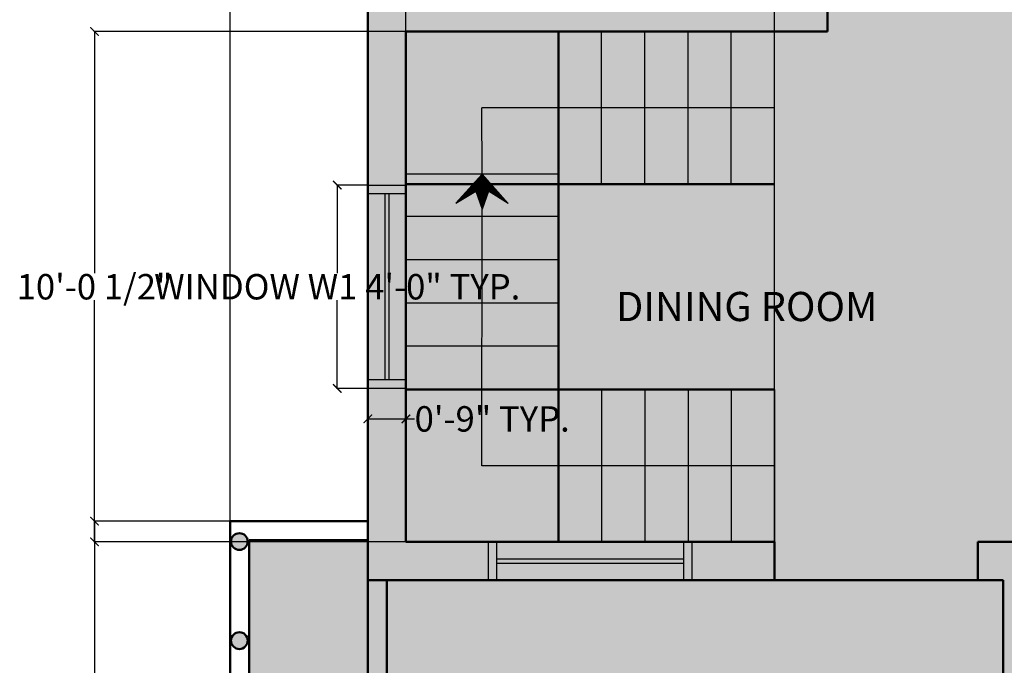
# Model space of a CAD drawing. Units: inches. Extents: x 528 to 2620, y -1066 to 798.
# Tile 22 of 41: x 975 to 1207, y 371 to 524. Entities that reach past the tile are written whole.
import ezdxf

# ---------------------------------------------------------------- set-up
doc = ezdxf.new("R2010")
doc.units = ezdxf.units.IN
doc.header["$MEASUREMENT"] = 0
for name, color, linetype, lineweight in [('A-ANNO-DIMS', 2, 'Continuous', 18), ('A-AREA-IDEN', 7, 'Continuous', 18), ('A-FLOR-STRS', 6, 'Continuous', 25), ('A-GLAZ', 3, 'Continuous', 25), ('A-WALL', 7, 'Continuous', 50), ('A-WALL-PATT', 8, 'Continuous', 13)]:
    doc.layers.add(name, color=color, linetype=linetype, lineweight=lineweight)
doc.styles.get("Standard").update_dxf_attribs({"font": 'arial.ttf'})
doc.dimstyles.get("Standard").update_dxf_attribs({"dimtxt": 6, "dimasz": 2, "dimexe": 0.18, "dimexo": 0.0625, "dimgap": 0.09, "dimtad": 0, "dimtih": 1, "dimtoh": 1, "dimdec": 1, "dimzin": 0, "dimdsep": 46, "dimlunit": 3, "dimtxsty": 'Standard', "dimblk": 'ARCHTICK', "dimcen": 0.09, "dimadec": 0, "dimazin": 0, "dimtfac": 1, "dimtdec": 1, "dimtofl": 0, "dimtmove": 0, "dimatfit": 3, "dimfxl": 1, "dimtolj": 1, "dimtzin": 0, "dimarcsym": 0})

# ---------------------------------------------------------------- blocks, each defined once
blk = doc.blocks.new('WIN-1200')
for p, q in [((677.56, 718.92), (725.56, 718.92)), ((677.56, 709.92), (677.56, 718.92)), ((679.56, 709.92), (679.56, 718.92)), ((723.56, 718.92), (723.56, 709.92)), ((725.56, 718.92), (725.56, 709.92)), ((679.56, 714.92), (723.56, 714.92)), ((679.56, 713.92), (723.56, 713.92)), ((725.56, 709.92), (677.56, 709.92))]:
    blk.add_line(p, q)
blk = doc.blocks.new('_ArchTick')
at = {"color": 0, "linetype": 'ByBlock', "const_width": 0.15}
blk.add_lwpolyline([(-0.5, -0.5), (0.5, 0.5)], dxfattribs=at)
blk = doc.blocks.new('*D50')
at = {"layer": 'A-ANNO-DIMS', "color": 0, "lineweight": -2, "transparency": 16777216}
for p, q in [((1056.93, 484.67), (1049.62, 484.67)), ((1049.8, 484.67), (1049.8, 463.87)), ((1049.8, 436.67), (1049.8, 457.48)), ((1056.93, 436.67), (1049.62, 436.67))]:
    blk.add_line(p, q, dxfattribs=at)
at = {"layer": 'Defpoints', "color": 0, "transparency": 16777216}
for p in [(1057, 484.67), (1049.8, 436.67), (1057, 436.67)]:
    blk.add_point(p, dxfattribs=at)
at = {"layer": 'A-ANNO-DIMS', "color": 0, "lineweight": -2, "transparency": 16777216, "xscale": 2, "yscale": 2, "zscale": 2}
for p, rotation in [((1049.8, 484.67), 90), ((1049.8, 436.67), 270)]:
    blk.add_blockref('_ArchTick', p, dxfattribs=dict(at, rotation=rotation))
at = {"layer": 'A-ANNO-DIMS', "color": 0, "transparency": 16777216, "insert": (1049.8, 460.67), "char_height": 6, "attachment_point": 5}
blk.add_mtext('\\A1;WINDOW W1 4\'-0" TYP.', dxfattribs=at)
blk = doc.blocks.new('*D51')
at = {"layer": 'A-ANNO-DIMS', "color": 0, "lineweight": -2, "transparency": 16777216}
for p, q in [((1057, 436.61), (1057, 429.29)), ((1066, 436.61), (1066, 429.29)), ((1057, 429.47), (1066, 429.47)), ((1066, 429.47), (1068, 429.47))]:
    blk.add_line(p, q, dxfattribs=at)
at = {"layer": 'Defpoints', "color": 0, "transparency": 16777216}
for p in [(1057, 436.67), (1066, 436.67), (1066, 429.47)]:
    blk.add_point(p, dxfattribs=at)
at = {"layer": 'A-ANNO-DIMS', "color": 0, "lineweight": -2, "transparency": 16777216, "xscale": 2, "yscale": 2, "zscale": 2, "rotation": 180}
blk.add_blockref('_ArchTick', (1057, 429.47), dxfattribs=at)
at = {"layer": 'A-ANNO-DIMS', "color": 0, "lineweight": -2, "transparency": 16777216, "xscale": 2, "yscale": 2, "zscale": 2}
blk.add_blockref('_ArchTick', (1066, 429.47), dxfattribs=at)
at = {"layer": 'A-ANNO-DIMS', "color": 0, "transparency": 16777216, "insert": (1086.37, 429.47), "char_height": 6, "attachment_point": 5}
blk.add_mtext('\\A1;0\'-9" TYP.', dxfattribs=at)
blk = doc.blocks.new('*D63')
at = {"layer": 'A-ANNO-DIMS', "color": 0, "lineweight": -2, "transparency": 16777216}
for p, q in [((1024.5, 405.4), (1024.5, 751.1)), ((1024.5, 750.92), (1025.64, 750.92)), ((1057, 750.92), (1055.85, 750.92)), ((1057, 405.4), (1057, 751.1))]:
    blk.add_line(p, q, dxfattribs=at)
at = {"layer": 'Defpoints', "color": 0, "transparency": 16777216}
for p in [(1057, 750.92), (1024.5, 405.34), (1057, 405.34)]:
    blk.add_point(p, dxfattribs=at)
at = {"layer": 'A-ANNO-DIMS', "color": 0, "lineweight": -2, "transparency": 16777216, "xscale": 2, "yscale": 2, "zscale": 2, "rotation": 180}
blk.add_blockref('_ArchTick', (1024.5, 750.92), dxfattribs=at)
at = {"layer": 'A-ANNO-DIMS', "color": 0, "lineweight": -2, "transparency": 16777216, "xscale": 2, "yscale": 2, "zscale": 2}
blk.add_blockref('_ArchTick', (1057, 750.92), dxfattribs=at)
at = {"layer": 'A-ANNO-DIMS', "color": 0, "transparency": 16777216, "insert": (1040.75, 750.92), "char_height": 6, "attachment_point": 5}
blk.add_mtext('\\A1;2\'-8 1/2"', dxfattribs=at)
blk = doc.blocks.new('*D64')
at = {"layer": 'A-ANNO-DIMS', "color": 0, "lineweight": -2, "transparency": 16777216}
for p, q in [((1024.43, 405.34), (992.32, 405.34)), ((992.5, 405.34), (992.5, 320.03)), ((992.5, 228.42), (992.5, 313.73)), ((1024.43, 228.42), (992.32, 228.42))]:
    blk.add_line(p, q, dxfattribs=at)
at = {"layer": 'Defpoints', "color": 0, "transparency": 16777216}
for p in [(1024.5, 405.34), (992.5, 228.42), (1024.5, 228.42)]:
    blk.add_point(p, dxfattribs=at)
at = {"layer": 'A-ANNO-DIMS', "color": 0, "lineweight": -2, "transparency": 16777216, "xscale": 2, "yscale": 2, "zscale": 2}
for p, rotation in [((992.5, 405.34), 90), ((992.5, 228.42), 270)]:
    blk.add_blockref('_ArchTick', p, dxfattribs=dict(at, rotation=rotation))
at = {"layer": 'A-ANNO-DIMS', "color": 0, "transparency": 16777216, "insert": (992.5, 316.88), "char_height": 6, "attachment_point": 5}
blk.add_mtext('\\A1;14\'-9"', dxfattribs=at)
blk = doc.blocks.new('*D66')
at = {"layer": 'A-ANNO-DIMS', "color": 0, "lineweight": -2, "transparency": 16777216}
for p, q in [((1066, 400.48), (1066, 751.1)), ((1066, 750.92), (1101.46, 750.92)), ((1153, 750.92), (1117.54, 750.92)), ((1153, 400.48), (1153, 751.1))]:
    blk.add_line(p, q, dxfattribs=at)
at = {"layer": 'Defpoints', "color": 0, "transparency": 16777216}
for p in [(1153, 750.92), (1066, 400.42), (1153, 400.42)]:
    blk.add_point(p, dxfattribs=at)
at = {"layer": 'A-ANNO-DIMS', "color": 0, "lineweight": -2, "transparency": 16777216, "xscale": 2, "yscale": 2, "zscale": 2, "rotation": 180}
blk.add_blockref('_ArchTick', (1066, 750.92), dxfattribs=at)
at = {"layer": 'A-ANNO-DIMS', "color": 0, "lineweight": -2, "transparency": 16777216, "xscale": 2, "yscale": 2, "zscale": 2}
blk.add_blockref('_ArchTick', (1153, 750.92), dxfattribs=at)
at = {"layer": 'A-ANNO-DIMS', "color": 0, "transparency": 16777216, "insert": (1109.5, 750.92), "char_height": 6, "attachment_point": 5}
blk.add_mtext('\\A1;7\'-3"', dxfattribs=at)
blk = doc.blocks.new('*D67')
at = {"layer": 'A-ANNO-DIMS', "color": 0, "lineweight": -2, "transparency": 16777216}
for p, q in [((1152.93, 520.92), (992.32, 520.92)), ((992.5, 520.92), (992.5, 463.86)), ((992.5, 400.42), (992.5, 457.48)), ((1152.93, 400.42), (992.32, 400.42))]:
    blk.add_line(p, q, dxfattribs=at)
at = {"layer": 'Defpoints', "color": 0, "transparency": 16777216}
for p in [(1153, 520.92), (992.5, 400.42), (1153, 400.42)]:
    blk.add_point(p, dxfattribs=at)
at = {"layer": 'A-ANNO-DIMS', "color": 0, "lineweight": -2, "transparency": 16777216, "xscale": 2, "yscale": 2, "zscale": 2}
for p, rotation in [((992.5, 520.92), 90), ((992.5, 400.42), 270)]:
    blk.add_blockref('_ArchTick', p, dxfattribs=dict(at, rotation=rotation))
at = {"layer": 'A-ANNO-DIMS', "color": 0, "transparency": 16777216, "insert": (992.5, 460.67), "char_height": 6, "attachment_point": 5}
blk.add_mtext('\\A1;10\'-0 1/2"', dxfattribs=at)

msp = doc.modelspace()

# ---------------------------------------------------------------- hatches: boundary and pattern name
at = {"layer": 'A-GLAZ', "transparency": 33554687}
h = msp.add_hatch(color=256, dxfattribs=at)
h.dxf.hatch_style = 1
h.paths.add_polyline_path([(1061.5, 391.42), (1057, 391.42), (1057, 307.96), (1061.5, 307.96)])
h.paths.add_polyline_path([(1081, 305.42), (1069, 305.42), (1069, 300.92), (1081, 300.92)])
h.paths.add_polyline_path([(1141, 305.42), (1129, 305.42), (1129, 300.92), (1141, 300.92)])
h.paths.add_polyline_path([(1207, 305.42), (1201, 305.42), (1201, 300.92), (1207, 300.92)])
at = {"layer": 'A-WALL-PATT', "transparency": 33554521}
h = msp.add_hatch(color=256, dxfattribs=at)
h.dxf.hatch_style = 1
h.paths.add_polyline_path([(1066, 709.92), (1114.5, 709.92), (1114.5, 718.92), (1057, 718.92), (1057, 667.92), (1066, 667.92)])
h.paths.add_polyline_path([(1227.5, 718.92), (1162.5, 718.92), (1162.5, 709.92), (1211, 709.92), (1211, 577.92), (1205.42, 577.92), (1205.5, 573.42), (1211, 573.42), (1211, 567.42), (1215.5, 567.42), (1215.5, 669.42), (1268, 669.42), (1268, 675.92), (1263.5, 675.92), (1263.5, 673.92), (1215.5, 673.92), (1215.5, 709.92), (1227.5, 709.92)])
h.paths.add_polyline_path([(1345, 718.92), (1316, 718.92), (1316, 709.92), (1336, 709.92), (1336, 641.67), (1345, 641.67)])
h.paths.add_polyline_path([(1066, 619.92), (1057, 619.92), (1057, 561.42), (1066, 561.42), (1066, 573.42), (1161, 573.42), (1161, 569.42), (1165.5, 569.42), (1165.5, 577.92), (1066, 577.92)])
h.paths.add_polyline_path([(1216, 391.42), (1216, 400.42), (1207, 400.42), (1201, 400.42), (1201, 397.42), (1201, 391.42), (1207, 391.42), (1207, 268.92), (1252, 268.92), (1252, 277.92), (1216, 277.92), (1216, 359.77)])
h.paths.add_polyline_path([(1345, 395.92), (1336, 395.92), (1288, 395.92), (1288, 391.42), (1336, 391.42), (1336, 277.92), (1300, 277.92), (1300, 268.92), (1345, 268.92)])
h.paths.add_polyline_path([(1345, 593.67), (1336, 593.67), (1336, 525.42), (1215.5, 525.42), (1215.5, 527.17), (1211, 527.17), (1211, 520.92), (1336, 520.92), (1336, 443.92), (1345, 443.92)])
h.paths.add_polyline_path([(1066, 520.92), (1165.5, 520.92), (1165.5, 545.42), (1161, 545.42), (1161, 525.42), (1066, 525.42), (1066, 537.42), (1057, 537.42), (1057, 484.67), (1066, 484.67)])
h.paths.add_polyline_path([(1066, 436.67), (1057, 436.67), (1057, 391.42), (1085.5, 391.42), (1085.5, 400.42), (1066, 400.42)])
h.paths.add_polyline_path([(1153, 397.42), (1153, 400.42), (1133.5, 400.42), (1133.5, 391.42), (1153, 391.42)])
at = {"layer": 'A-WALL-PATT', "transparency": 33554681}
h = msp.add_hatch(color=256, dxfattribs=at)
h.dxf.hatch_style = 1
h.paths.add_polyline_path([(1062, 665.92), (1061, 665.92), (1061, 621.92), (1062, 621.92)])
h.paths.add_polyline_path([(1066, 667.92), (1057, 667.92), (1057, 665.92), (1066, 665.92)])
h.paths.add_polyline_path([(1066, 621.92), (1057, 621.92), (1057, 619.92), (1066, 619.92)])
h.paths.add_polyline_path([(1160.5, 714.92), (1116.5, 714.92), (1116.5, 713.92), (1160.5, 713.92)])
h.paths.add_polyline_path([(1162.5, 718.92), (1160.5, 718.92), (1160.5, 709.92), (1162.5, 709.92)])
h.paths.add_polyline_path([(1116.5, 718.92), (1114.5, 718.92), (1114.5, 709.92), (1116.5, 709.92)])
h.paths.add_polyline_path([(1251.5, 714.92), (1227.5, 714.92), (1227.5, 713.92), (1251.5, 713.92)])
h.paths.add_polyline_path([(1314, 714.92), (1270, 714.92), (1270, 713.92), (1314, 713.92)])
h.paths.add_polyline_path([(1316, 718.92), (1314, 718.92), (1314, 709.92), (1316, 709.92)])
h.paths.add_polyline_path([(1270, 718.92), (1268, 718.92), (1268, 709.92), (1270, 709.92)])
h.paths.add_polyline_path([(1087.5, 400.42), (1085.5, 400.42), (1085.5, 391.42), (1087.5, 391.42)])
h.paths.add_polyline_path([(1131.5, 396.42), (1087.5, 396.42), (1087.5, 395.42), (1131.5, 395.42)])
h.paths.add_polyline_path([(1133.5, 400.42), (1131.5, 400.42), (1131.5, 391.42), (1133.5, 391.42)])
h.paths.add_polyline_path([(1066, 438.67), (1057, 438.67), (1057, 436.67), (1066, 436.67)])
h.paths.add_polyline_path([(1066, 484.67), (1057, 484.67), (1057, 482.67), (1066, 482.67)])
h.paths.add_polyline_path([(1062, 482.67), (1061, 482.67), (1061, 438.67), (1062, 438.67)])
h = msp.add_hatch(color=256, dxfattribs=at)
h.dxf.hatch_style = 1
h.paths.add_polyline_path([(1066, 665.92), (1062, 665.92), (1062, 621.92), (1066, 621.92)])
h.paths.add_polyline_path([(1061, 665.92), (1057, 665.92), (1057, 621.92), (1061, 621.92)])
h.paths.add_polyline_path([(1160.5, 713.92), (1116.5, 713.92), (1116.5, 709.92), (1160.5, 709.92)])
h.paths.add_polyline_path([(1160.5, 718.92), (1116.5, 718.92), (1116.5, 714.92), (1160.5, 714.92)])
h.paths.add_polyline_path([(1251.5, 713.92), (1227.5, 713.92), (1227.5, 709.92), (1251.5, 709.92)])
h.paths.add_polyline_path([(1251.5, 718.92), (1227.5, 718.92), (1227.5, 714.92), (1251.5, 714.92)])
h.paths.add_polyline_path([(1314, 713.92), (1270, 713.92), (1270, 709.92), (1314, 709.92)])
h.paths.add_polyline_path([(1314, 718.92), (1270, 718.92), (1270, 714.92), (1314, 714.92)])
h.paths.add_polyline_path([(1345, 639.67), (1341, 639.67), (1341, 595.67), (1345, 595.67)])
h.paths.add_polyline_path([(1340, 639.67), (1336, 639.67), (1336, 595.67), (1340, 595.67)])
h.paths.add_polyline_path([(1345, 441.92), (1341, 441.92), (1341, 397.92), (1345, 397.92)])
h.paths.add_polyline_path([(1340, 441.92), (1336, 441.92), (1336, 397.92), (1340, 397.92)])
h.paths.add_polyline_path([(1298, 272.92), (1254, 272.92), (1254, 268.92), (1298, 268.92)])
h.paths.add_polyline_path([(1298, 277.92), (1254, 277.92), (1254, 273.92), (1298, 273.92)])
h.paths.add_polyline_path([(1131.5, 395.42), (1087.5, 395.42), (1087.5, 391.42), (1131.5, 391.42)])
h.paths.add_polyline_path([(1131.5, 400.42), (1087.5, 400.42), (1087.5, 396.42), (1131.5, 396.42)])
h.paths.add_polyline_path([(1066, 482.67), (1062, 482.67), (1062, 438.67), (1066, 438.67)])
h.paths.add_polyline_path([(1061, 482.67), (1057, 482.67), (1057, 438.67), (1061, 438.67)])
h.paths.add_polyline_path([(1066, 561.42), (1062, 561.42), (1062, 537.42), (1066, 537.42)])
h.paths.add_polyline_path([(1061, 561.42), (1057, 561.42), (1057, 537.42), (1061, 537.42)])
at = {"layer": 'A-WALL-PATT', "transparency": 33554536}
h = msp.add_hatch(color=256, dxfattribs=at)
h.dxf.hatch_style = 1
h.paths.add_polyline_path([(1336, 709.92), (1268, 709.92), (1268, 699.92), (1266.75, 699.92), (1266.75, 675.92), (1268, 675.92), (1268, 669.42), (1215.5, 669.42), (1215.5, 567.17), (1217, 567.17), (1257, 567.17), (1257, 565.42), (1256.96, 565.42, -0.401453), (1217, 527.17), (1215.5, 527.17), (1215.5, 525.42), (1336, 525.42)], flags=17)
h.paths.add_polyline_path([(1285.03, 635.93), (1285.23, 636.13), (1285.67, 636.26), (1286.21, 636.02), (1286.98, 636.08), (1332.98, 636.08), (1333.36, 636.22), (1333.82, 636.08), (1334.11, 635.71), (1334.11, 635.3), (1333.91, 634.86), (1333.82, 634.83), (1333.82, 592.74), (1333.97, 592.6), (1334.11, 592.29), (1334.11, 591.88), (1333.82, 591.51), (1333.36, 591.37), (1332.98, 591.51), (1332.64, 591.79), (1332.64, 591.51), (1286.98, 591.51), (1286.17, 591.67), (1286.07, 591.57), (1285.68, 591.37), (1285.23, 591.51), (1285.03, 591.71), (1284.83, 592.1), (1284.98, 592.54), (1285.13, 592.69), (1285.13, 634.95), (1284.98, 635.1), (1284.83, 635.54)], flags=16)
h.paths.add_polyline_path([(1285.03, 635.93), (1285.23, 636.13), (1285.67, 636.26), (1286.21, 636.02), (1286.98, 636.08), (1332.98, 636.08), (1333.36, 636.22), (1333.82, 636.08), (1334.11, 635.71), (1334.11, 635.3), (1333.97, 634.99), (1333.82, 634.85), (1333.82, 592.74), (1333.97, 592.6), (1334.11, 592.29), (1334.11, 591.88), (1333.82, 591.51), (1333.36, 591.37), (1332.98, 591.51), (1332.64, 591.79), (1332.64, 592.25), (1332.64, 635.35), (1332.64, 635.8), (1332.98, 636.08), (1312.23, 636.08), (1311.1, 635.48), (1310.63, 635.48), (1310.43, 635.23), (1309.94, 635.1), (1309.7, 634.99), (1309.06, 634.76), (1308.71, 634.61), (1308.32, 634.61), (1307.75, 634.36), (1307.11, 634.27), (1307.01, 634.11), (1306.77, 634.02), (1307.25, 633.28), (1306.87, 633.04), (1306.77, 632.88), (1306.37, 632.64), (1306.03, 632.55), (1305.54, 632.41), (1315.47, 618.49), (1316.32, 619.39), (1312.77, 622.86), (1319.62, 630.11), (1320.07, 629.68), (1320.11, 630), (1320.28, 630.6), (1320.53, 631.18), (1320.53, 632.01), (1320.26, 632.55), (1320.11, 633.13), (1320.06, 633.73), (1320.63, 634.02), (1321.22, 634.16), (1321.86, 634.11), (1322.45, 633.91), (1322.99, 633.62), (1324.1, 633.62), (1324.64, 633.91), (1325.23, 634.07), (1325.87, 634.07), (1326.43, 633.91), (1326.98, 633.62), (1328.35, 633.62), (1328.9, 633.91), (1329.49, 634.11), (1330.1, 634.16), (1330.69, 634.02), (1331.28, 633.73), (1331.23, 633.13), (1331.09, 632.55), (1330.79, 632.01), (1330.79, 631.18), (1331.04, 630.6), (1331.23, 630), (1331.28, 629.41), (1331.19, 628.79), (1331.04, 628.18), (1330.79, 627.6), (1330.79, 626.77), (1331.04, 626.19), (1331.23, 625.59), (1331.28, 625.01), (1331.19, 624.38), (1331.04, 623.78), (1330.79, 623.24), (1330.79, 622.37), (1331.04, 621.83), (1331.23, 621.25), (1331.28, 620.6), (1331.19, 619.97), (1331.04, 619.37), (1330.79, 618.83), (1330.79, 617.96), (1331.09, 617.42), (1331.23, 616.88), (1331.28, 616.23), (1331.28, 615.52), (1330.69, 615.27), (1330.1, 615.12), (1329.49, 615.12), (1328.9, 615.32), (1328.35, 615.65), (1326.98, 615.65), (1326.43, 615.32), (1325.87, 615.16), (1325.23, 615.16), (1324.64, 615.32), (1324.1, 615.65), (1323.24, 615.65), (1324.93, 614.04), (1322.98, 611.98), (1324.1, 611.98), (1324.64, 612.27), (1325.28, 612.43), (1325.87, 612.43), (1326.48, 612.27), (1327.03, 611.98), (1328.35, 611.98), (1328.9, 612.27), (1329.49, 612.48), (1330.1, 612.52), (1330.74, 612.39), (1331.28, 612.07), (1331.28, 611.36), (1331.28, 610.75), (1331.09, 610.17), (1330.79, 609.63), (1330.79, 608.81), (1331.09, 608.22), (1331.23, 607.62), (1331.28, 606.99), (1331.23, 606.41), (1331.09, 605.81), (1330.79, 605.22), (1330.79, 604.4), (1331.09, 603.81), (1331.23, 603.21), (1331.28, 602.63), (1331.23, 602), (1331.09, 601.4), (1330.79, 600.86), (1330.79, 599.99), (1331.09, 599.45), (1331.23, 598.87), (1331.28, 598.22), (1331.23, 597.59), (1331.09, 596.99), (1330.79, 596.45), (1330.79, 595.58), (1331.09, 595.04), (1331.28, 594.51), (1331.28, 593.86), (1330.74, 593.61), (1330.1, 593.48), (1329.49, 593.48), (1328.9, 593.68), (1328.35, 594.01), (1327.03, 594.01), (1326.48, 593.68), (1325.87, 593.52), (1325.28, 593.52), (1324.64, 593.68), (1324.1, 594.01), (1323.04, 594.01), (1322.5, 593.68), (1321.91, 593.48), (1321.27, 593.48), (1320.63, 593.61), (1320.11, 593.86), (1320.11, 594.51), (1320.28, 595.04), (1320.58, 595.58), (1320.58, 596.45), (1320.28, 596.99), (1320.16, 597.59), (1320.1, 598.01), (1319.62, 597.55), (1315.66, 601.73), (1312.23, 591.57), (1311.74, 591.66), (1311.59, 591.91), (1310.78, 592.4), (1309.55, 592.89), (1308.96, 592.89), (1308.71, 593.03), (1308.56, 593.14), (1307.75, 593.52), (1306.77, 593.61), (1307.25, 594.36), (1306.87, 594.6), (1306.37, 594.84), (1306.03, 595.09), (1305.54, 595.24), (1315.46, 609.35), (1310.93, 613.71), (1315.47, 618.49), (1305.54, 632.41), (1306.03, 632.55), (1306.37, 632.64), (1306.77, 632.88), (1306.87, 633.04), (1307.25, 633.28), (1306.77, 634.02), (1307.01, 634.11), (1307.11, 634.27), (1307.75, 634.36), (1308.32, 634.61), (1308.71, 634.61), (1309.06, 634.76), (1309.7, 634.99), (1309.94, 635.1), (1310.43, 635.23), (1310.63, 635.48), (1311.1, 635.48), (1312.23, 636.08), (1286.98, 636.08), (1286.22, 636.02), (1286.41, 635.44), (1286.21, 635.05), (1286.02, 634.85), (1285.87, 634.81), (1285.87, 592.84), (1286.15, 592.73), (1286.41, 592.19), (1286.23, 591.66), (1286.17, 591.67), (1286.07, 591.57), (1285.68, 591.37), (1285.23, 591.51), (1285.03, 591.71), (1284.83, 592.1), (1284.98, 592.54), (1285.13, 592.69), (1285.13, 634.95), (1284.98, 635.1), (1284.83, 635.54)], flags=0)
h.paths.add_polyline_path([(1322.5, 653.6), (1333.65, 653.6), (1333.65, 637.99), (1322.5, 637.99)], flags=16)
h.paths.add_polyline_path([(1323.62, 652.48), (1332.53, 652.48), (1332.53, 639.11), (1323.62, 639.11)], flags=0)
edge = h.paths.add_edge_path(flags=0)
edge.add_ellipse((1328.07, 645.79), major_axis=(2.24, 2.24), ratio=1, start_angle=405, end_angle=495, ccw=False)
edge.add_ellipse((1328.07, 645.79), major_axis=(2.24, 2.24), ratio=1, start_angle=675, end_angle=765, ccw=False)
edge.add_ellipse((1328.07, 645.79), major_axis=(2.24, 2.24), ratio=1, start_angle=585, end_angle=675, ccw=False)
edge.add_ellipse((1328.07, 645.79), major_axis=(2.24, 2.24), ratio=1, start_angle=495, end_angle=585, ccw=False)
h.paths.add_polyline_path([(1320.58, 628.39), (1320.33, 628.01), (1320.61, 628.55)], flags=0)
h.paths.add_polyline_path([(1317.89, 604.89), (1318.78, 604.64), (1319.76, 604.28), (1318.88, 604.53)], flags=0)
h.paths.add_polyline_path([(1320.33, 599.65), (1320.58, 599.25), (1320.58, 599.16)], flags=0)
h.paths.add_polyline_path([(1322.5, 589.6), (1333.65, 589.6), (1333.65, 573.99), (1322.5, 573.99)], flags=16)
h.paths.add_polyline_path([(1323.62, 588.48), (1332.53, 588.48), (1332.53, 575.11), (1323.62, 575.11)], flags=0)
edge = h.paths.add_edge_path(flags=0)
edge.add_ellipse((1328.07, 581.8), major_axis=(-2.24, 2.24), ratio=1, start_angle=-45, end_angle=45, ccw=False)
edge.add_ellipse((1328.07, 581.8), major_axis=(-2.24, 2.24), ratio=1, start_angle=-135, end_angle=-45, ccw=False)
edge.add_ellipse((1328.07, 581.8), major_axis=(-2.24, 2.24), ratio=1, start_angle=135, end_angle=-135, ccw=False)
edge.add_ellipse((1328.07, 581.8), major_axis=(-2.24, 2.24), ratio=1, start_angle=45, end_angle=135, ccw=False)
h.paths.add_polyline_path([(1264.75, 699.92), (1263.5, 699.92), (1263.5, 709.92), (1215.5, 709.92), (1215.5, 673.92), (1263.5, 673.92), (1263.5, 675.92), (1264.75, 675.92)], flags=16)
h.paths.add_polyline_path([(1162.19, 569.42), (1161, 569.42), (1161, 573.42), (1066, 573.42), (1066, 525.42), (1161, 525.42), (1161, 545.42), (1162.19, 545.42)])
h.paths.add_polyline_path([(1256.96, 565.42), (1257, 565.42), (1257, 567.17), (1217, 567.17), (1215.5, 567.17), (1215.5, 567.42), (1211, 567.42), (1211, 573.42), (1205.5, 573.42), (1205.42, 577.92), (1211, 577.92), (1211, 709.92), (1066, 709.92), (1066, 577.92), (1165.5, 577.92), (1165.5, 569.42), (1164.19, 569.42), (1164.19, 545.42), (1165.5, 545.42), (1165.5, 520.92), (1153, 520.92), (1153, 484.92), (1102, 484.92), (1102, 436.42), (1153, 436.42), (1153, 400.42), (1153, 391.42), (1201, 391.42), (1201, 400.42), (1207, 400.42), (1216, 400.42), (1216, 391.42), (1216, 277.92), (1336, 277.92), (1336, 391.42), (1288, 391.42), (1288, 395.92), (1336, 395.92), (1336, 443.92), (1336, 520.92), (1211, 520.92), (1211, 527.17), (1215.5, 527.17), (1217, 527.17, 0.401453)])
h.paths.add_polyline_path([(1167.25, 579.42), (1165.5, 579.42), (1165.5, 619.42), (1167.25, 619.42)], flags=16)
h.paths.add_polyline_path([(1227.97, 501.56), (1236.36, 502.03), (1236.36, 492.55), (1227.97, 493.02, -0.254069)], flags=16)
h.paths.add_polyline_path([(1243.34, 515.69, -0.254069), (1251.88, 515.69), (1252.35, 507.3), (1242.87, 507.3)], flags=16)
h.paths.add_polyline_path([(1239.18, 504.68), (1256.03, 504.68), (1256.03, 479.42), (1239.18, 479.42)], flags=16)
h.paths.add_polyline_path([(1227.97, 489.6), (1236.36, 490.07), (1236.36, 480.59), (1227.97, 481.06, -0.254069)], flags=16)
h.paths.add_polyline_path([(1197.2, 624.04), (1197.2, 639.64), (1208.35, 639.64), (1208.35, 624.04)], flags=16)
h.paths.add_polyline_path([(1198.32, 625.15), (1198.32, 638.53), (1207.23, 638.53), (1207.23, 625.15)], flags=0)
h.paths.add_polyline_path([(1258.85, 502.03), (1267.25, 501.56, -0.254069), (1267.25, 493.02), (1258.85, 492.55)], flags=16)
h.paths.add_polyline_path([(1271.59, 519.66), (1333.67, 519.66), (1333.67, 451.59), (1319.09, 451.59), (1319.09, 505.07), (1288.09, 505.07), (1284.45, 505.07, -0.883215), (1270.68, 514.19), (1270.68, 518.75, -0.414214)], flags=16)
h.paths.add_polyline_path([(1331.85, 517.83), (1331.85, 453.42), (1328.2, 453.42), (1328.2, 505.07), (1298.42, 505.07), (1298.42, 514.19), (1288.09, 514.19), (1288.09, 517.83)], flags=0)
h.paths.add_polyline_path([(1242.87, 476.8), (1252.35, 476.8), (1251.88, 468.41, -0.254069), (1243.34, 468.41)], flags=16)
h.paths.add_polyline_path([(1258.85, 490.07), (1267.25, 489.6, -0.254069), (1267.25, 481.06), (1258.85, 480.59)], flags=16)
h.paths.add_polyline_path([(1161.68, 641.55), (1160.87, 641.72), (1160.77, 641.62), (1160.38, 641.41), (1159.93, 641.55), (1159.73, 641.75), (1159.53, 642.14), (1159.68, 642.58), (1159.83, 642.73), (1159.83, 684.99), (1159.68, 685.14), (1159.53, 685.58), (1159.73, 685.97), (1159.93, 686.17), (1160.37, 686.31), (1160.91, 686.06), (1161.68, 686.13), (1207.68, 686.13), (1208.06, 686.27), (1208.52, 686.13), (1208.81, 685.76), (1208.81, 685.34), (1208.61, 684.9), (1208.52, 684.87), (1208.52, 642.78), (1208.67, 642.65), (1208.88, 642.2), (1208.72, 641.8), (1208.52, 641.55), (1208.06, 641.41), (1207.68, 641.55), (1207.34, 641.83), (1207.34, 641.55)], flags=16)
h.paths.add_polyline_path([(1186.93, 641.62), (1186.44, 641.71), (1186.29, 641.95), (1185.48, 642.45), (1184.25, 642.94), (1183.66, 642.94), (1183.41, 643.07), (1183.26, 643.18), (1182.45, 643.57), (1181.47, 643.65), (1181.95, 644.4), (1181.57, 644.64), (1181.07, 644.89), (1180.73, 645.13), (1180.24, 645.29), (1190.16, 659.4), (1185.63, 663.75), (1190.17, 668.54), (1180.24, 682.46), (1180.73, 682.59), (1181.07, 682.68), (1181.47, 682.93), (1181.57, 683.08), (1181.95, 683.33), (1181.47, 684.07), (1181.71, 684.16), (1181.81, 684.31), (1182.45, 684.4), (1183.02, 684.65), (1183.41, 684.65), (1183.76, 684.81), (1184.4, 685.03), (1184.64, 685.14), (1185.13, 685.28), (1185.33, 685.52), (1185.8, 685.52), (1186.93, 686.13), (1161.68, 686.13), (1160.92, 686.06), (1161.11, 685.49), (1160.91, 685.1), (1160.72, 684.9), (1160.57, 684.85), (1160.57, 642.88), (1160.85, 642.77), (1161.11, 642.23), (1160.93, 641.7), (1160.87, 641.72), (1160.77, 641.62), (1160.38, 641.41), (1159.93, 641.55), (1159.73, 641.75), (1159.53, 642.14), (1159.68, 642.58), (1159.83, 642.73), (1159.83, 684.99), (1159.68, 685.14), (1159.53, 685.58), (1159.73, 685.97), (1159.93, 686.17), (1160.37, 686.31), (1160.91, 686.06), (1161.68, 686.13), (1207.68, 686.13), (1208.06, 686.27), (1208.52, 686.13), (1208.81, 685.76), (1208.81, 685.34), (1208.67, 685.03), (1208.52, 684.9), (1208.52, 642.78), (1208.67, 642.65), (1208.88, 642.2), (1208.72, 641.8), (1208.52, 641.55), (1208.06, 641.41), (1207.68, 641.55), (1207.34, 641.83), (1207.34, 642.29), (1207.34, 685.39), (1207.34, 685.85), (1207.68, 686.13), (1186.93, 686.13), (1185.8, 685.52), (1185.33, 685.52), (1185.13, 685.28), (1184.64, 685.14), (1184.4, 685.03), (1183.76, 684.81), (1183.41, 684.65), (1183.02, 684.65), (1182.45, 684.4), (1181.81, 684.31), (1181.71, 684.16), (1181.47, 684.07), (1181.95, 683.33), (1181.57, 683.08), (1181.47, 682.93), (1181.07, 682.68), (1180.73, 682.59), (1180.24, 682.46), (1190.17, 668.54), (1191.02, 669.43), (1187.47, 672.9), (1194.32, 680.15), (1194.77, 679.72), (1194.81, 680.04), (1194.98, 680.65), (1195.23, 681.23), (1195.23, 682.05), (1194.96, 682.59), (1194.81, 683.17), (1194.76, 683.78), (1195.33, 684.07), (1195.92, 684.2), (1196.56, 684.16), (1197.15, 683.96), (1197.69, 683.67), (1198.8, 683.67), (1199.34, 683.96), (1199.93, 684.11), (1200.57, 684.11), (1201.13, 683.96), (1201.68, 683.67), (1203.05, 683.67), (1203.6, 683.96), (1204.19, 684.16), (1204.8, 684.2), (1205.39, 684.07), (1205.98, 683.78), (1205.93, 683.17), (1205.79, 682.59), (1205.49, 682.05), (1205.49, 681.23), (1205.74, 680.65), (1205.93, 680.04), (1205.98, 679.46), (1205.89, 678.83), (1205.74, 678.23), (1205.49, 677.65), (1205.49, 676.82), (1205.74, 676.24), (1205.93, 675.63), (1205.98, 675.05), (1205.89, 674.42), (1205.74, 673.82), (1205.49, 673.28), (1205.49, 672.41), (1205.74, 671.87), (1205.93, 671.29), (1205.98, 670.64), (1205.89, 670.02), (1205.74, 669.41), (1205.49, 668.87), (1205.49, 668), (1205.79, 667.46), (1205.93, 666.93), (1205.98, 666.28), (1205.98, 665.56), (1205.39, 665.32), (1204.8, 665.16), (1204.19, 665.16), (1203.6, 665.36), (1203.05, 665.7), (1201.68, 665.7), (1201.13, 665.36), (1200.57, 665.2), (1199.93, 665.2), (1199.34, 665.36), (1198.8, 665.7), (1197.94, 665.7), (1199.63, 664.09), (1197.68, 662.03), (1198.8, 662.03), (1199.34, 662.32), (1199.98, 662.47), (1200.57, 662.47), (1201.18, 662.32), (1201.73, 662.03), (1203.05, 662.03), (1203.6, 662.32), (1204.19, 662.52), (1204.8, 662.56), (1205.44, 662.43), (1205.98, 662.12), (1205.98, 661.4), (1205.98, 660.8), (1205.79, 660.21), (1205.49, 659.68), (1205.49, 658.85), (1205.79, 658.27), (1205.93, 657.66), (1205.98, 657.04), (1205.93, 656.45), (1205.79, 655.85), (1205.49, 655.27), (1205.49, 654.44), (1205.79, 653.86), (1205.93, 653.25), (1205.98, 652.67), (1205.93, 652.05), (1205.79, 651.44), (1205.49, 650.91), (1205.49, 650.03), (1205.79, 649.5), (1205.93, 648.91), (1205.98, 648.26), (1205.93, 647.64), (1205.79, 647.03), (1205.49, 646.5), (1205.49, 645.62), (1205.79, 645.09), (1205.98, 644.55), (1205.98, 643.9), (1205.44, 643.65), (1204.8, 643.52), (1204.19, 643.52), (1203.6, 643.72), (1203.05, 644.06), (1201.73, 644.06), (1201.18, 643.72), (1200.57, 643.57), (1199.98, 643.57), (1199.34, 643.72), (1198.8, 644.06), (1197.74, 644.06), (1197.2, 643.72), (1196.61, 643.52), (1195.97, 643.52), (1195.33, 643.65), (1194.81, 643.9), (1194.81, 644.55), (1194.98, 645.09), (1195.28, 645.62), (1195.28, 646.5), (1194.98, 647.03), (1194.86, 647.64), (1194.8, 648.06), (1194.32, 647.59), (1190.36, 651.77)], flags=16)
h.paths.add_polyline_path([(1195.28, 649.2), (1195.03, 649.7), (1195.28, 649.29)], flags=0)
h.paths.add_polyline_path([(1194.46, 654.33), (1193.58, 654.58), (1192.59, 654.93), (1193.48, 654.69)], flags=0)
h.paths.add_polyline_path([(1195.28, 678.43), (1195.03, 678.05), (1195.31, 678.59)], flags=0)
h.paths.add_polyline_path([(1197.2, 688.04), (1197.2, 703.64), (1208.35, 703.64), (1208.35, 688.04)], flags=16)
h.paths.add_polyline_path([(1198.32, 689.15), (1198.32, 702.53), (1207.23, 702.53), (1207.23, 689.15)], flags=0)
h.paths.add_polyline_path([(1217.1, 329.02), (1230.65, 329.02), (1230.65, 315.47), (1217.1, 315.47)], flags=16)
h.paths.add_polyline_path([(1223.87, 322.24), (1227.26, 322.24), (1227.26, 321.32, -0.414214), (1229.73, 318.86, -1), (1224.8, 318.86), (1223.87, 318.86)], flags=0)
h.paths.add_polyline_path([(1222.11, 325.63, -1), (1218.86, 325.63, -1)], flags=0)
h.paths.add_polyline_path([(1228.25, 325.63, -1), (1226.28, 325.63, -1)], flags=0)
h.paths.add_polyline_path([(1221.53, 318.86, -1), (1219.44, 318.86, -1)], flags=0)
h.paths.add_polyline_path([(1299.15, 293.73), (1299.15, 278.54), (1271.23, 278.54), (1271.23, 293.73)], flags=16)
h.paths.add_polyline_path([(1259.69, 292.21), (1270.62, 292.21, -1), (1270.62, 291.6), (1259.69, 291.6, -1)], flags=16)
h.paths.add_polyline_path([(1259.69, 291.3), (1270.62, 291.3, -1), (1270.62, 290.69), (1259.69, 290.69, -1)], flags=16)
h.paths.add_polyline_path([(1259.69, 290.39), (1270.62, 290.39, -1), (1270.62, 289.78), (1259.69, 289.78, -1)], flags=16)
h.paths.add_polyline_path([(1259.69, 289.48), (1270.62, 289.48, -1), (1270.62, 288.87), (1259.69, 288.87, -1)], flags=16)
h.paths.add_polyline_path([(1259.69, 288.57), (1270.62, 288.57, -1), (1270.62, 287.96), (1259.69, 287.96, -1)], flags=16)
h.paths.add_polyline_path([(1274.41, 292.38), (1283.25, 292.38, -0.414214), (1285.07, 290.56), (1285.07, 283.64, -0.414214), (1283.25, 281.82), (1277.72, 281.82), (1278.67, 280.87, -0.57735), (1279.38, 280.16), (1279.44, 280.11, -1), (1279.03, 279.7), (1278.97, 279.75, -0.57735), (1278.26, 280.46), (1276.9, 281.82), (1274.41, 281.82, -0.414214), (1272.58, 283.64), (1272.58, 290.56, -0.414214)], flags=0)
h.paths.add_polyline_path([(1259.69, 287.65), (1270.62, 287.65, -1), (1270.62, 287.05), (1259.69, 287.05, -1)], flags=16)
h.paths.add_polyline_path([(1259.69, 286.74), (1270.62, 286.74, -1), (1270.62, 286.14), (1259.69, 286.14, -1)], flags=16)
h.paths.add_polyline_path([(1259.69, 285.83), (1270.62, 285.83, -1), (1270.62, 285.22), (1259.69, 285.22, -1)], flags=16)
h.paths.add_polyline_path([(1259.69, 284.92), (1270.62, 284.92, -1), (1270.62, 284.31), (1259.69, 284.31, -1)], flags=16)
h.paths.add_polyline_path([(1259.69, 284.01), (1270.62, 284.01, -1), (1270.62, 283.4), (1259.69, 283.4, -1)], flags=16)
h.paths.add_polyline_path([(1287.82, 292.38), (1296.67, 292.38, -0.414214), (1298.49, 290.56), (1298.49, 283.64, -0.414214), (1296.67, 281.82), (1291.14, 281.82), (1292.09, 280.87, -0.57735), (1292.8, 280.16), (1292.85, 280.11, -1), (1292.44, 279.7), (1292.39, 279.75, -0.57735), (1291.68, 280.46), (1290.32, 281.82), (1287.82, 281.82, -0.414214), (1286, 283.64), (1286, 290.56, -0.414214)], flags=0)
h.paths.add_polyline_path([(1259.69, 283.1), (1270.62, 283.1, -1), (1270.62, 282.49), (1259.69, 282.49, -1)], flags=16)
h.paths.add_polyline_path([(1279.94, 287.61, -1), (1278.01, 287.61, -1)], flags=0)
h.paths.add_polyline_path([(1259.69, 282.19), (1270.62, 282.19, -1), (1270.62, 281.58), (1259.69, 281.58, -1)], flags=16)
h.paths.add_polyline_path([(1259.69, 281.27), (1270.62, 281.27, -1), (1270.62, 280.67), (1259.69, 280.67, -1)], flags=16)
h.paths.add_polyline_path([(1275.16, 284.17, -1), (1274.77, 284.17, -1)], flags=0)
h.paths.add_polyline_path([(1293.36, 287.61, -1), (1291.43, 287.61, -1)], flags=0)
h.paths.add_polyline_path([(1275.14, 280.5), (1276.33, 280.5, -5.828427), (1276.33, 280.12), (1275.14, 280.12, -1)], flags=0)
h.paths.add_polyline_path([(1288.57, 284.17, -1), (1288.19, 284.17, -1)], flags=0)
h.paths.add_polyline_path([(1281.31, 280.5), (1282.5, 280.5, -1), (1282.5, 280.12), (1281.31, 280.12, -5.828427)], flags=0)
h.paths.add_polyline_path([(1288.56, 280.5), (1289.75, 280.5, -5.828427), (1289.75, 280.12), (1288.56, 280.12, -1)], flags=0)
h.paths.add_polyline_path([(1294.73, 280.5), (1295.92, 280.5, -1), (1295.92, 280.12), (1294.73, 280.12, -5.828427)], flags=0)
h.paths.add_polyline_path([(1207, 391.42), (1201, 391.42), (1061.5, 391.42), (1061.5, 307.96), (1069, 307.96), (1069, 305.42), (1207, 305.42)])
h = msp.add_hatch(color=256, dxfattribs=at)
h.dxf.hatch_style = 1
h.paths.add_polyline_path([(1102, 436.42), (1083.93, 436.42), (1083.9, 418.42), (1102, 418.42)], flags=17)
h.paths.add_polyline_path([(1102, 418.42), (1083.9, 418.42), (1083.93, 436.42), (1066, 436.42), (1066, 400.42), (1102, 400.42)])
h.paths.add_polyline_path([(1122.4, 436.42), (1112.2, 436.42), (1112.2, 418.42), (1122.4, 418.42)])
h.paths.add_polyline_path([(1122.4, 418.42), (1112.2, 418.42), (1112.2, 400.42), (1122.4, 400.42)])
h.paths.add_polyline_path([(1112.2, 418.42), (1102, 418.42), (1102, 400.42), (1112.2, 400.42)])
h.paths.add_polyline_path([(1112.2, 436.42), (1102, 436.42), (1102, 418.42), (1112.2, 418.42)])
h.paths.add_polyline_path([(1132.6, 436.42), (1122.4, 436.42), (1122.4, 418.42), (1132.6, 418.42)])
h.paths.add_polyline_path([(1132.6, 418.42), (1122.4, 418.42), (1122.4, 400.42), (1132.6, 400.42)])
h.paths.add_polyline_path([(1142.8, 418.42), (1132.6, 418.42), (1132.6, 400.42), (1133.5, 400.42), (1142.8, 400.42)])
h.paths.add_polyline_path([(1142.8, 436.42), (1132.6, 436.42), (1132.6, 418.42), (1142.8, 418.42)])
h.paths.add_polyline_path([(1153, 436.42), (1142.8, 436.42), (1142.8, 418.42), (1153, 418.42)])
h.paths.add_polyline_path([(1153, 418.42), (1142.8, 418.42), (1142.8, 400.42), (1153, 400.42)])
h.paths.add_polyline_path([(1083.94, 446.62), (1066, 446.62), (1066, 436.67), (1066, 436.42), (1083.93, 436.42)])
h.paths.add_polyline_path([(1102, 446.62), (1083.94, 446.62), (1083.93, 436.42), (1102, 436.42)])
h.paths.add_polyline_path([(1102, 456.82), (1083.96, 456.82), (1083.94, 446.62), (1102, 446.62)])
h.paths.add_polyline_path([(1083.96, 456.82), (1066, 456.82), (1066, 446.62), (1083.94, 446.62)])
h.paths.add_polyline_path([(1083.97, 467.02), (1066, 467.02), (1066, 456.82), (1083.96, 456.82)])
h.paths.add_polyline_path([(1102, 467.02), (1083.97, 467.02), (1083.96, 456.82), (1102, 456.82)])
h.paths.add_polyline_path([(1102, 477.22), (1083.98, 477.22), (1083.97, 467.02), (1102, 467.02)])
h.paths.add_polyline_path([(1083.98, 477.22), (1066, 477.22), (1066, 467.02), (1083.97, 467.02)])
h.paths.add_polyline_path([(1083.99, 479.02), (1082.47, 483.25), (1077.81, 480.37), (1081.92, 484.92), (1066, 484.92), (1066, 477.22), (1083.98, 477.22)])
h.paths.add_polyline_path([(1102, 484.92), (1086.06, 484.92), (1090.16, 480.35), (1085.51, 483.24), (1083.99, 479.02), (1083.98, 477.22), (1102, 477.22)])
h.paths.add_polyline_path([(1102, 487.22), (1084, 487.22), (1086.06, 484.92), (1102, 484.92)])
h.paths.add_polyline_path([(1084, 487.22), (1066, 487.22), (1066, 484.92), (1081.92, 484.92)])
h.paths.add_polyline_path([(1083.9, 502.92), (1102, 502.92), (1102, 520.92), (1066, 520.92), (1066, 487.22), (1084, 487.22)])
h.paths.add_polyline_path([(1102, 502.92), (1083.9, 502.92), (1084, 487.22), (1102, 487.22)])
h.paths.add_polyline_path([(1122.4, 520.92), (1112.2, 520.92), (1112.2, 502.92), (1122.4, 502.92)])
h.paths.add_polyline_path([(1122.4, 502.92), (1112.2, 502.92), (1112.2, 484.92), (1122.4, 484.92)])
h.paths.add_polyline_path([(1112.2, 502.92), (1102, 502.92), (1102, 487.22), (1102, 484.92), (1112.2, 484.92)])
h.paths.add_polyline_path([(1112.2, 520.92), (1102, 520.92), (1102, 502.92), (1112.2, 502.92)])
h.paths.add_polyline_path([(1132.6, 520.92), (1122.4, 520.92), (1122.4, 502.92), (1132.6, 502.92)])
h.paths.add_polyline_path([(1132.6, 502.92), (1122.4, 502.92), (1122.4, 484.92), (1132.6, 484.92)])
h.paths.add_polyline_path([(1142.8, 502.92), (1132.6, 502.92), (1132.6, 484.92), (1142.8, 484.92)])
h.paths.add_polyline_path([(1142.8, 520.92), (1132.6, 520.92), (1132.6, 502.92), (1142.8, 502.92)])
h.paths.add_polyline_path([(1153, 520.92), (1142.8, 520.92), (1142.8, 502.92), (1153, 502.92)])
h.paths.add_polyline_path([(1153, 502.92), (1142.8, 502.92), (1142.8, 484.92), (1153, 484.92)])
at = {"layer": 'A-WALL-PATT'}
h = msp.add_hatch(dxfattribs=at)
h.set_pattern_fill('ANSI31', color=256)
h.set_pattern_definition([(45, (436.937, 0), (-0.088388348, 0.088388348), [])])
h.paths.add_polyline_path([(1084, 487.22), (1077.81, 480.37), (1082.47, 483.25), (1083.99, 479.02), (1085.51, 483.24), (1090.16, 480.35)])
at = {"layer": 'A-WALL-PATT', "transparency": 33554687}
h = msp.add_hatch(color=256, dxfattribs=at)
h.dxf.hatch_style = 1
h.paths.add_polyline_path([(1024.71, 400.5, 1), (1028.67, 400.5, 1)])
at = {"layer": 'A-WALL-PATT', "transparency": 33554536}
h = msp.add_hatch(color=256, dxfattribs=at)
h.dxf.hatch_style = 1
h.paths.add_polyline_path([(1207, 300.92), (1069, 300.92), (1069, 298.96), (1057, 298.96), (1057, 307.96), (1057, 391.42), (1057, 400.84), (1029, 400.84), (1029, 232.92), (1207, 232.92), (1207, 268.92)])
at = {"layer": 'A-WALL-PATT', "transparency": 33554687}
h = msp.add_hatch(color=256, dxfattribs=at)
h.dxf.hatch_style = 1
h.paths.add_polyline_path([(1024.71, 377.12, 1), (1028.67, 377.12, 1)])

# ---------------------------------------------------------------- linework, layer by layer
at = {"layer": 'A-FLOR-STRS'}
for p, q in [((1112.2, 484.92), (1112.2, 520.92)), ((1112.2, 484.92), (1112.2, 520.92)), ((1122.4, 484.92), (1122.4, 520.92)), ((1122.4, 484.92), (1122.4, 520.92)), ((1132.6, 484.92), (1132.6, 520.92)), ((1132.6, 484.92), (1132.6, 520.92)), ((1142.8, 484.92), (1142.8, 520.92)), ((1142.8, 484.92), (1142.8, 520.92)), ((1153, 484.92), (1153, 520.92)), ((1153, 484.92), (1153, 520.92)), ((1153, 502.92), (1083.9, 502.92)), ((1153, 502.92), (1083.9, 502.92)), ((1084, 487.22), (1083.9, 502.92)), ((1102, 487.22), (1066, 487.22)), ((1084, 487.22), (1077.81, 480.37)), ((1084, 487.22), (1090.16, 480.35)), ((1077.81, 480.37), (1082.47, 483.25)), ((1082.47, 483.25), (1083.99, 479.02)), ((1085.51, 483.24), (1083.99, 479.02)), ((1090.16, 480.35), (1085.51, 483.24)), ((1083.9, 418.42), (1083.99, 479.02)), ((1102, 477.22), (1066, 477.22)), ((1102, 467.02), (1066, 467.02)), ((1102, 456.82), (1066, 456.82)), ((1102, 446.62), (1066, 446.62)), ((1102, 436.42), (1066, 436.42)), ((1102, 436.42), (1102, 400.42)), ((1112.2, 436.42), (1112.2, 400.42)), ((1112.2, 436.42), (1112.2, 400.42)), ((1122.4, 436.42), (1122.4, 400.42)), ((1122.4, 436.42), (1122.4, 400.42)), ((1132.6, 436.42), (1132.6, 400.42)), ((1132.6, 436.42), (1132.6, 400.42)), ((1142.8, 436.42), (1142.8, 400.42)), ((1142.8, 436.42), (1142.8, 400.42)), ((1153, 436.42), (1153, 400.42)), ((1153, 436.42), (1153, 400.42)), ((1153, 418.42), (1083.9, 418.42)), ((1153, 418.42), (1083.9, 418.42))]:
    msp.add_line(p, q, dxfattribs=at)
at = {"layer": 'A-WALL'}
for p, q in [((1057, 718.92), (1057, 391.42)), ((1165.5, 545.42), (1165.5, 520.92)), ((1165.5, 520.92), (1066, 520.92)), ((1066, 520.92), (1066, 400.42)), ((1102, 520.92), (1102, 400.42)), ((1153, 484.92), (1066, 484.92)), ((1153, 484.92), (1066, 484.92)), ((1153, 436.42), (1066, 436.42)), ((1153, 436.42), (1066, 436.42)), ((1024.5, 405.34), (1024.5, 228.42)), ((1057, 405.34), (1024.5, 405.34)), ((1057, 400.84), (1029, 400.84)), ((1029, 400.84), (1029, 232.92)), ((1153, 400.42), (1066, 400.42)), ((1153, 391.42), (1153, 400.42)), ((1207, 400.42), (1201, 400.42)), ((1201, 391.42), (1201, 400.42)), ((1216, 400.42), (1207, 400.42)), ((1153, 391.42), (1057, 391.42)), ((1057, 391.42), (1201, 391.42)), ((1057, 391.42), (1057, 300.92)), ((1061.5, 391.42), (1061.5, 305.42)), ((1207, 391.42), (1201, 391.42)), ((1201, 391.42), (1207, 391.42)), ((1207, 268.92), (1207, 391.42)), ((1207, 391.42), (1207, 268.92))]:
    msp.add_line(p, q, dxfattribs=at)
for centre in [(1026.69, 400.5), (1026.69, 377.12)]:
    msp.add_circle(centre, 1.98, dxfattribs=at)

# ---------------------------------------------------------------- block references
at = {"layer": 'A-GLAZ', "rotation": 269.9999999999996}
msp.add_blockref('WIN-1200', (347.07, 1162.23), dxfattribs=at)
at = {"layer": 'A-GLAZ'}
msp.add_blockref('WIN-1200', (407.94, -318.5), dxfattribs=at)

# ---------------------------------------------------------------- texts
at = {"layer": 'A-AREA-IDEN'}
msp.add_text('DINING ROOM', height=6.8907, dxfattribs=at).set_placement((1115.58, 452.56))

# ---------------------------------------------------------------- dimensions: what is measured, and where the dimension line sits
at = {"layer": 'A-ANNO-DIMS'}
for base, p1, p2, picture, middle in [((1057, 750.92), (1024.5, 405.34), (1057, 405.34), '*D63', (1040.75, 750.92)), ((1153, 750.92), (1066, 400.42), (1153, 400.42), '*D66', (1109.5, 750.92))]:
    dim = msp.add_linear_dim(base=base, p1=p1, p2=p2, dimstyle='Standard', override={"dimdec": 1, "dimlfac": 1, "dimrnd": 0, "dimzin": 1, "dimdsep": 46, "dimlunit": 4, "dimfrac": 2}, dxfattribs=at)
    dim.commit()
    dim.dimension.update_dxf_attribs({"geometry": picture, "text_midpoint": middle})
for base, p1, p2, picture, middle in [((992.5, 400.42), (1153, 520.92), (1153, 400.42), '*D67', (992.5, 460.67)), ((992.5, 228.42), (1024.5, 405.34), (1024.5, 228.42), '*D64', (992.5, 316.88))]:
    dim = msp.add_linear_dim(base=base, p1=p1, p2=p2, angle=90, dimstyle='Standard', override={"dimdec": 1, "dimlfac": 1, "dimrnd": 0, "dimzin": 1, "dimdsep": 46, "dimlunit": 4, "dimfrac": 2}, dxfattribs=at)
    dim.commit()
    dim.dimension.update_dxf_attribs({"geometry": picture, "text_midpoint": middle})
dim = msp.add_linear_dim(base=(1049.8, 436.67), p1=(1057, 484.67), p2=(1057, 436.67), angle=270, text='WINDOW W1 <> TYP.', dimstyle='Standard', override={"dimdec": 1, "dimrnd": 0, "dimzin": 1, "dimlunit": 4, "dimfrac": 2}, dxfattribs=at)
dim.commit()
dim.dimension.update_dxf_attribs({"geometry": '*D50', "text_midpoint": (1049.8, 460.67)})
dim = msp.add_linear_dim(base=(1066, 429.47), p1=(1057, 436.67), p2=(1066, 436.67), text='<> TYP.', dimstyle='Standard', override={"dimdec": 1, "dimrnd": 0, "dimzin": 1, "dimlunit": 4, "dimfrac": 2}, dxfattribs=at)
dim.commit()
dim.dimension.update_dxf_attribs({"geometry": '*D51', "text_midpoint": (1086.37, 429.47)})

doc.saveas('drawing.dxf')
